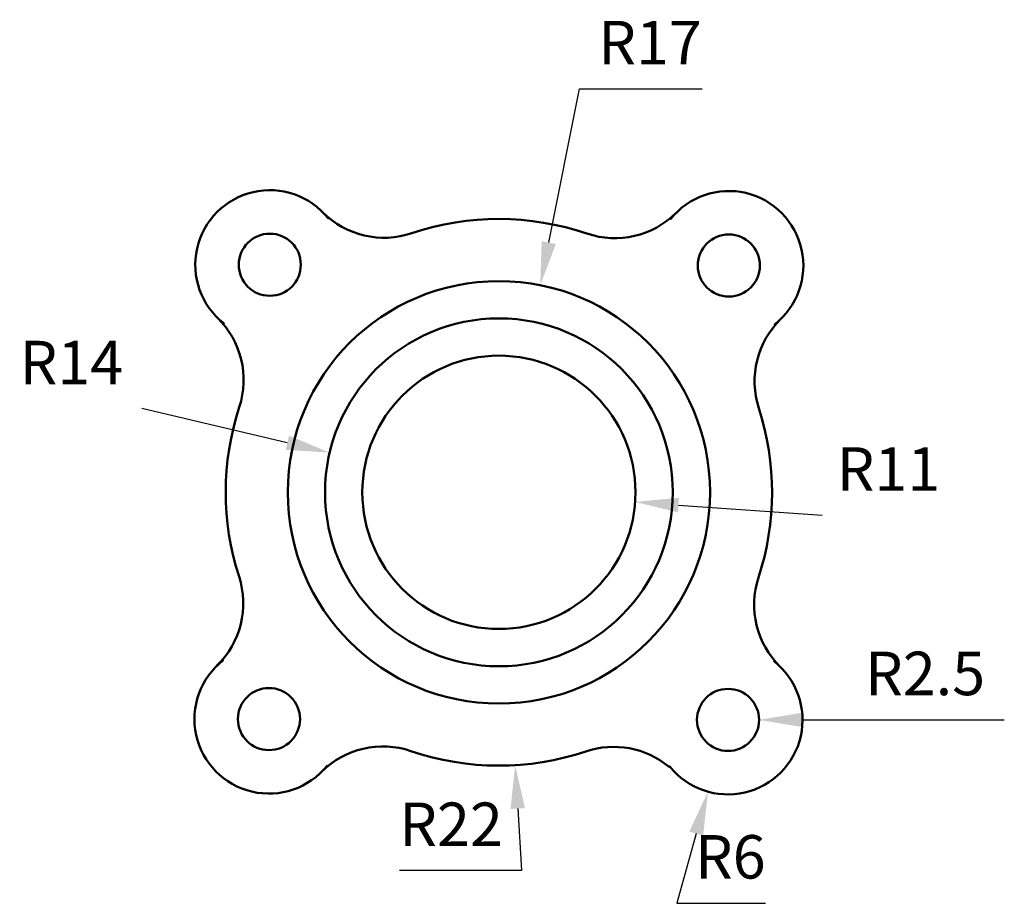
# Model space of a CAD drawing. Units: millimetres. Extents: x 142.6 to 221.9, y 113 to 184.1.
import ezdxf

# ---------------------------------------------------------------- set-up
doc = ezdxf.new("R2010")
doc.units = ezdxf.units.MM
doc.layers.add('M-DIMS', color=3, linetype='Continuous', lineweight=25)
doc.layers.add('M-OUTL', color=7, linetype='Continuous', lineweight=50)
doc.styles.get("Standard").update_dxf_attribs({"font": 'arial.ttf'})
doc.dimstyles.new('AM_ISO$4', dxfattribs={"dimtxt": 3.5, "dimasz": 3.5, "dimexe": 1, "dimexo": 1, "dimgap": 1.5, "dimtad": 1, "dimtoh": 1, "dimdsep": 46, "dimtxsty": 'Standard', "dimcen": 0, "dimclrd": 256, "dimclre": 256, "dimclrt": 2, "dimadec": 0, "dimazin": 2, "dimtp": 0.1, "dimtm": 0.1, "dimtfac": 0.71, "dimtdec": 3, "dimtofl": 0, "dimtmove": 0, "dimatfit": 0, "dimfxl": 1, "dimlwd": -1, "dimlwe": -1, "dimarcsym": 1})

# ---------------------------------------------------------------- blocks, each defined once
blk = doc.blocks.new('*D3')
at = {"layer": 'Defpoints', "color": 0, "transparency": 16777216}
for p in [(199.685, 127.761), (198.067, 121.984)]:
    blk.add_point(p, dxfattribs=at)
at = {"layer": 'M-DIMS', "color": 0, "linetype": 'ByBlock', "transparency": 16777216}
for p, q in [((197.124, 118.613), (195.551, 112.999)), ((195.551, 112.999), (202.693, 112.999))]:
    blk.add_line(p, q, dxfattribs=at)
at = {"layer": 'M-DIMS', "color": 0, "transparency": 16777216}
blk.add_solid([(196.562, 118.771), (197.685, 118.456), (198.067, 121.984)], dxfattribs=at)
at = {"layer": 'M-DIMS', "color": 0, "transparency": 16777216, "insert": (199.872, 116.286), "char_height": 3.5, "attachment_point": 5}
blk.add_mtext('R6', dxfattribs=at)
blk = doc.blocks.new('*D4')
at = {"layer": 'Defpoints', "color": 0, "transparency": 16777216}
for p in [(199.685, 127.761), (202.185, 127.761)]:
    blk.add_point(p, dxfattribs=at)
at = {"layer": 'M-DIMS', "color": 0, "linetype": 'ByBlock', "transparency": 16777216}
blk.add_line((205.685, 127.761), (221.933, 127.761), dxfattribs=at)
at = {"layer": 'M-DIMS', "color": 0, "transparency": 16777216}
blk.add_solid([(205.685, 128.345), (205.685, 127.178), (202.185, 127.761)], dxfattribs=at)
at = {"layer": 'M-DIMS', "color": 0, "transparency": 16777216, "insert": (215.559, 131.048), "char_height": 3.5, "attachment_point": 5}
blk.add_mtext('R2.5', dxfattribs=at)
blk = doc.blocks.new('*D5')
at = {"layer": 'Defpoints', "color": 0, "transparency": 16777216}
for p in [(181.235, 146.081), (182.544, 124.12)]:
    blk.add_point(p, dxfattribs=at)
at = {"layer": 'M-DIMS', "color": 0, "linetype": 'ByBlock', "transparency": 16777216}
for p, q in [((182.752, 120.626), (183.049, 115.649)), ((183.049, 115.649), (173.221, 115.649))]:
    blk.add_line(p, q, dxfattribs=at)
at = {"layer": 'M-DIMS', "color": 0, "transparency": 16777216}
blk.add_solid([(183.334, 120.661), (182.17, 120.591), (182.544, 124.12)], dxfattribs=at)
at = {"layer": 'M-DIMS', "color": 0, "transparency": 16777216, "insert": (177.385, 118.906), "char_height": 3.5, "attachment_point": 5}
blk.add_mtext('R22', dxfattribs=at)
blk = doc.blocks.new('*D6')
at = {"layer": 'Defpoints', "color": 0, "transparency": 16777216}
for p in [(184.567, 162.751), (181.235, 146.081)]:
    blk.add_point(p, dxfattribs=at)
at = {"layer": 'M-DIMS', "color": 0, "linetype": 'ByBlock', "transparency": 16777216}
for p, q in [((185.252, 166.183), (187.727, 178.569)), ((187.727, 178.569), (197.591, 178.569))]:
    blk.add_line(p, q, dxfattribs=at)
at = {"layer": 'M-DIMS', "color": 0, "transparency": 16777216}
blk.add_solid([(184.68, 166.298), (185.824, 166.069), (184.567, 162.751)], dxfattribs=at)
at = {"layer": 'M-DIMS', "color": 0, "transparency": 16777216, "insert": (193.409, 181.826), "char_height": 3.5, "attachment_point": 5}
blk.add_mtext('R17', dxfattribs=at)
blk = doc.blocks.new('*D7')
at = {"layer": 'Defpoints', "color": 0, "transparency": 16777216}
for p in [(167.604, 149.274), (181.235, 146.081)]:
    blk.add_point(p, dxfattribs=at)
at = {"layer": 'M-DIMS', "color": 0, "linetype": 'ByBlock', "transparency": 16777216}
blk.add_line((164.197, 150.072), (152.487, 152.814), dxfattribs=at)
at = {"layer": 'M-DIMS', "color": 0, "transparency": 16777216}
blk.add_solid([(164.33, 150.64), (164.064, 149.504), (167.604, 149.274)], dxfattribs=at)
at = {"layer": 'M-DIMS', "color": 0, "transparency": 16777216, "insert": (146.813, 156.071), "char_height": 3.5, "attachment_point": 5}
blk.add_mtext('R14', dxfattribs=at)
blk = doc.blocks.new('*D8')
at = {"layer": 'Defpoints', "color": 0, "transparency": 16777216}
for p in [(181.235, 146.081), (192.208, 145.305)]:
    blk.add_point(p, dxfattribs=at)
at = {"layer": 'M-DIMS', "color": 0, "linetype": 'ByBlock', "transparency": 16777216}
blk.add_line((195.699, 145.058), (207.266, 144.24), dxfattribs=at)
at = {"layer": 'M-DIMS', "color": 0, "transparency": 16777216}
blk.add_solid([(195.74, 145.64), (195.658, 144.476), (192.208, 145.305)], dxfattribs=at)
at = {"layer": 'M-DIMS', "color": 0, "transparency": 16777216, "insert": (212.61, 147.497), "char_height": 3.5, "attachment_point": 5}
blk.add_mtext('R11', dxfattribs=at)

msp = doc.modelspace()

# ---------------------------------------------------------------- linework, layer by layer
at = {"layer": 'M-OUTL'}
for points in [[(167.536, 168.179, 0.000676), (167.476, 168.142, 1.122884), (159.077, 159.683, 0.000676), (159.041, 159.623)], [(203.479, 159.542, 0.000676), (203.443, 159.602, 1.122884), (195.075, 168.091, 0.000676), (195.016, 168.129)], [(167.038, 168.633, 0.28536), (174.229, 166.935, -0.164434), (188.318, 166.91, 0.28536), (195.515, 168.581)], [(158.532, 132.127, 0.28536), (160.307, 139.299, -0.158914), (160.332, 152.939, 0.28536), (158.583, 160.118)], [(203.939, 160.035, 0.28536), (202.164, 152.863, -0.158914), (202.139, 139.223, 0.28536), (203.888, 132.044)], [(158.991, 132.62, 0.000676), (159.028, 132.56, 1.122884), (167.396, 124.07, 0.000676), (167.455, 124.033)], [(203.43, 132.538, -0.000676), (203.393, 132.478, -1.122884), (194.995, 124.02, -0.000676), (194.935, 123.983, 0.259506), (188.242, 125.226, -0.164434), (174.153, 125.252, 0.28536), (166.956, 123.581)]]:
    msp.add_lwpolyline(points, format="xyb", dxfattribs=at)
for centre, radius in [((162.785, 164.4), 2.5), ((199.752, 164.333), 2.5), ((181.235, 146.081), 17), ((181.235, 146.081), 14), ((181.235, 146.081), 11), ((162.719, 127.829), 2.5), ((199.685, 127.761), 2.5)]:
    msp.add_circle(centre, radius, dxfattribs=at)

# ---------------------------------------------------------------- dimensions: what is measured, and where the dimension line sits
at = {"layer": 'M-DIMS'}
for center, mpoint, override, picture, middle in [((181.235, 146.081), (184.567, 162.751), {"dimclrd": 0, "dimclre": 0, "dimclrt": 0}, '*D6', (193.409, 178.569)), ((181.235, 146.081), (167.604, 149.274), {"dimclrd": 0, "dimclre": 0, "dimclrt": 0}, '*D7', (146.813, 152.814)), ((181.235, 146.081), (192.208, 145.305), {"dimclrd": 0, "dimclre": 0, "dimclrt": 0}, '*D8', (212.61, 144.24)), ((181.235, 146.081), (182.544, 124.12), {"dimpost": '', "dimclrd": 0, "dimclre": 0, "dimclrt": 0}, '*D5', (177.385, 115.649)), ((199.685, 127.761), (202.185, 127.761), {"dimclrd": 0, "dimclre": 0, "dimclrt": 0}, '*D4', (215.559, 127.761)), ((199.685, 127.761), (198.067, 121.984), {"dimpost": '', "dimclrd": 0, "dimclre": 0, "dimclrt": 0}, '*D3', (199.872, 112.999))]:
    dim = msp.add_radius_dim(center=center, mpoint=mpoint, dimstyle='AM_ISO$4', override=override, dxfattribs=at)
    dim.commit()
    dim.dimension.update_dxf_attribs({"geometry": picture, "text_midpoint": middle, "dimtype": 164})

doc.saveas('drawing.dxf')
